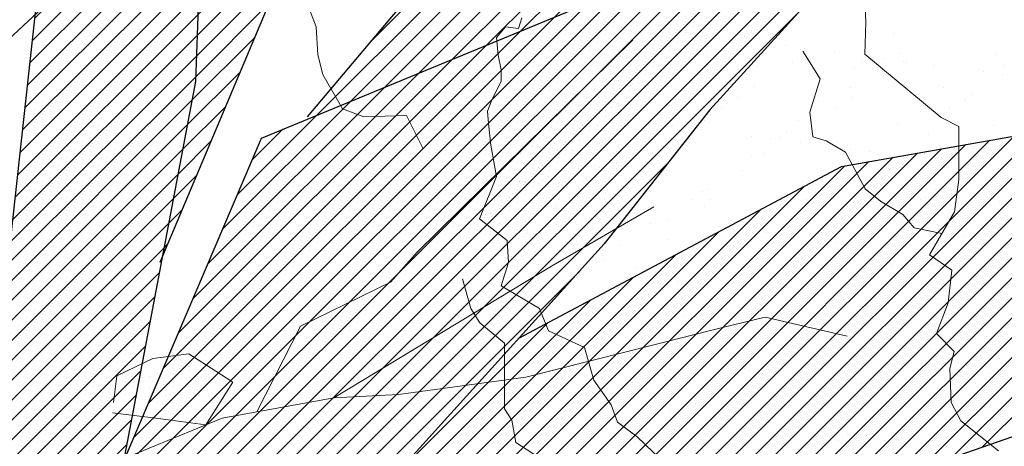
# Model space of a CAD drawing. Units: inches. Extents: x 1986 to 21484, y -1816 to 2016.
# Tile 32 of 85: x 2172.01 to 2182.74, y 1887.36 to 1892.02. Entities that reach past the tile are written whole.
import ezdxf

# ---------------------------------------------------------------- set-up
doc = ezdxf.new("R2010")
doc.units = ezdxf.units.IN
doc.layers.add('L-PLNT', color=84, linetype='Continuous', lineweight=13)
doc.layers.add('vfolhas', color=114, linetype='Continuous', lineweight=5)
doc.layers.add('vfolha2', color=110, linetype='Continuous')
doc.layers.add('vfolhas2', color=102, linetype='Continuous')
pattern_1 = [(45, (-2446.5133113, 50.986076), (-0.004419417382, 0.004419417382), [])]

# ---------------------------------------------------------------- blocks, each defined once
blk = doc.blocks.new('arbusto_PB_verde_grande')
at = {"layer": 'vfolha2'}
h = blk.add_hatch(dxfattribs=at)
h.set_pattern_fill('ANSI31', color=256, scale=0.05, style=0)
h.set_pattern_definition(pattern_1)
h.paths.add_polyline_path([(0.02944, 0.35651), (0.00028, 0.09048), (0.02625, -0.03934), (0.047, 0.06233), (0.06189, 0.09731), (0.09372, 0.26573), (0.09955, 0.43473), (0.08789, 0.61313), (0.0645, 0.72266), (0.04988, 0.6851), (0.0236, 0.51294)])
h.paths.add_polyline_path([(0.30106, 0.43789), (0.14225, 0.24871), (0.26685, 0.30022)])
h.paths.add_polyline_path([(0.37995, 0.22817), (0.23697, 0.15193), (0.18428, 0.09364), (0.11122, 0.04358), (0.02625, -0.03934), (0.28061, 0.04667), (0.36829, 0.07798), (0.46756, 0.11239), (0.61068, 0.19376), (0.71585, 0.27823), (0.55813, 0.25948)])
h.paths.add_polyline_path([(0.56101, -0.29441), (0.72752, -0.32573), (0.59024, -0.2412), (0.42962, -0.15982), (0.02625, -0.03934), (0.14922, -0.14107), (0.18838, -0.16604), (0.41501, -0.24435)])
h.paths.add_polyline_path([(-0.27429, -0.44776), (-0.30352, -0.72628), (-0.23923, -0.64175), (-0.15457, -0.45716), (0.02625, -0.03934), (-0.16328, -0.25376)])
h.paths.add_polyline_path([(-0.51963, -0.24744), (-0.67736, -0.32573), (-0.59558, -0.35072), (-0.40574, -0.32882), (-0.21007, -0.20995), (0.02625, -0.03934), (-0.14874, -0.06595), (-0.31518, -0.09101), (-0.41452, -0.15048)])
h.paths.add_polyline_path([(-0.52546, 0.25007), (-0.70947, 0.24698), (-0.51963, 0.1093), (-0.32979, 0.02167), (-0.07567, -0.0128), (-0.04234, -0.02148), (-0.35024, 0.1312)])
at = {"layer": 'vfolhas'}
h = blk.add_hatch(dxfattribs=at)
h.set_pattern_fill('ANSI31', color=256, scale=0.05, style=0)
h.set_pattern_definition(pattern_1)
h.paths.add_polyline_path([(-0.07279, 0.50669), (-0.18085, 0.65063), (-0.2334, 0.67253), (-0.20712, 0.53176), (-0.10785, 0.25007), (0.02625, -0.03934), (0.00028, 0.09048), (0.00816, 0.16241), (-0.04939, 0.29079)])
h.paths.add_polyline_path([(0.09902, 0.41929), (0.09372, 0.26573), (0.07906, 0.18814), (0.15506, 0.36901), (0.26606, 0.5505), (0.28356, 0.63504), (0.2485, 0.68819), (0.25145, 0.63504), (0.20178, 0.54426)])
h.paths.add_polyline_path([(0.12295, 0.24073), (0.047, 0.06233), (0.02625, -0.03934), (0.11122, 0.04358), (0.18428, 0.09364), (0.27478, 0.19376), (0.3215, 0.25323), (0.44129, 0.38467), (0.47634, 0.57866), (0.41789, 0.45347), (0.28939, 0.30954)])
h.paths.add_polyline_path([(0.58145, -0.03779), (0.70707, 0.01536), (0.78591, 0.04667), (0.74796, 0.06549), (0.62818, 0.08423), (0.52595, 0.09048), (0.39745, 0.04358), (0.02625, -0.03934), (0.25728, -0.03154), (0.43834, -0.0347)])
h.paths.add_polyline_path([(0.52022, -0.03647), (0.43834, -0.0347), (0.25728, -0.03154), (0.02625, -0.03934), (0.17964, -0.08515), (0.53768, -0.13167), (0.69541, -0.15357), (0.78591, -0.07852), (0.70413, -0.10042)])
h.paths.add_polyline_path([(0.27189, -0.21929), (0.14922, -0.14107), (0.02625, -0.03934), (0.15794, -0.31007), (0.29522, -0.42585), (0.41789, -0.49157), (0.56396, -0.56669), (0.5114, -0.48532), (0.39456, -0.34139)])
h.paths.add_polyline_path([(-0.05818, -0.47591), (-0.02312, -0.61984), (0.047, -0.80134), (0.08494, -0.59794), (0.07911, -0.4071), (0.03527, -0.25376), (0.02625, -0.03934), (-0.03773, -0.26001)])
h.paths.add_polyline_path([(-0.24218, 0.14054), (-0.11073, 0.06858), (0.02625, -0.03934), (-0.04235, 0.10871), (-0.21007, 0.23757), (-0.36485, 0.33145), (-0.47874, 0.40341), (-0.54303, 0.46288), (-0.49041, 0.33145), (-0.39408, 0.22192)])
at = {"layer": 'vfolha2'}
for p, q in [((0.14339, 0.25007), (0.30106, 0.43789)), ((0.09955, 0.43473), (0.09372, 0.26573)), ((0.00028, 0.09048), (0.02944, 0.35651)), ((0.37995, 0.22817), (0.55813, 0.25948)), ((0.23697, 0.15193), (0.37995, 0.22817))]:
    blk.add_line(p, q, dxfattribs=at)
at = {"layer": 'vfolhas2'}
for p, q in [((0.44129, 0.38467), (0.3215, 0.25323)), ((0.15506, 0.36901), (0.07795, 0.18551)), ((0.12295, 0.24073), (0.28939, 0.30954)), ((0.09372, 0.26573), (0.06189, 0.09731)), ((0.3215, 0.25323), (0.27478, 0.19376)), ((0.047, 0.06233), (0.12295, 0.24073)), ((0.27478, 0.19376), (0.18428, 0.09364)), ((0.46756, 0.11239), (0.36829, 0.07798))]:
    blk.add_line(p, q, dxfattribs=at)
blk = doc.blocks.new('PLANT-SHRUB')
for p, q in [((2171.837, 1891.752), (2172.54, 1892.411)), ((2175.047, 1892.46), (2175.244, 1891.941)), ((2181.225, 1892.278), (2181.234, 1891.991)), ((2177.484, 1892.037), (2177.448, 1891.922)), ((2178.209, 1892.018), (2178.209, 1892.018)), ((2178.417, 1891.991), (2178.417, 1891.991)), ((2178.742, 1891.948), (2178.742, 1891.948)), ((2181.234, 1891.991), (2181.225, 1891.643)), ((2175.244, 1891.941), (2175.262, 1891.636)), ((2177.307, 1891.939), (2177.209, 1891.824)), ((2177.448, 1891.922), (2177.307, 1891.939)), ((2178.292, 1891.909), (2178.292, 1891.909)), ((2178.568, 1891.93), (2178.568, 1891.93)), ((2178.681, 1891.891), (2178.681, 1891.891)), ((2178.722, 1891.865), (2178.722, 1891.865)), ((2178.789, 1891.908), (2178.789, 1891.908)), ((2179.285, 1891.877), (2179.285, 1891.877)), ((2179.493, 1891.849), (2179.493, 1891.849)), ((2179.91, 1891.837), (2179.91, 1891.837)), ((2179.984, 1891.904), (2179.984, 1891.904)), ((2181.533, 1891.872), (2181.533, 1891.872)), ((2176.344, 1889.483), (2178.697, 1891.799)), ((2177.209, 1891.824), (2177.227, 1891.63)), ((2178.689, 1891.748), (2178.689, 1891.748)), ((2179.818, 1891.807), (2179.818, 1891.807)), ((2180.361, 1891.735), (2180.361, 1891.735)), ((2175.262, 1891.636), (2175.316, 1891.422)), ((2177.227, 1891.63), (2177.262, 1891.471)), ((2178.558, 1891.622), (2178.558, 1891.622)), ((2179.503, 1891.686), (2179.503, 1891.686)), ((2180.525, 1891.691), (2180.525, 1891.691)), ((2180.736, 1891.375), (2180.547, 1891.676)), ((2180.569, 1891.708), (2180.569, 1891.708)), ((2180.894, 1891.665), (2180.894, 1891.665)), ((2181.225, 1891.643), (2182.057, 1890.952)), ((2181.604, 1891.652), (2181.604, 1891.652)), ((2182.651, 1891.639), (2182.651, 1891.639)), ((2179.193, 1891.557), (2179.193, 1891.557)), ((2180.438, 1891.555), (2180.438, 1891.555)), ((2181.185, 1891.553), (2181.185, 1891.553)), ((2181.437, 1891.593), (2181.437, 1891.593)), ((2181.645, 1891.566), (2181.645, 1891.566)), ((2181.682, 1891.553), (2181.682, 1891.553)), ((2181.97, 1891.523), (2181.97, 1891.523)), ((2182.734, 1891.521), (2182.734, 1891.521)), ((2175.316, 1891.422), (2175.531, 1891.046)), ((2177.262, 1891.471), (2177.262, 1891.347)), ((2178.593, 1891.464), (2178.593, 1891.464)), ((2178.66, 1891.507), (2178.66, 1891.507)), ((2178.764, 1891.464), (2178.764, 1891.464)), ((2179.512, 1891.472), (2179.512, 1891.472)), ((2181.112, 1891.486), (2181.112, 1891.486)), ((2182.512, 1891.452), (2182.512, 1891.452)), ((2182.72, 1891.424), (2182.72, 1891.424)), ((2177.262, 1891.347), (2177.156, 1891.135)), ((2178.328, 1891.382), (2178.328, 1891.382)), ((2178.411, 1891.371), (2178.411, 1891.371)), ((2178.541, 1891.354), (2178.541, 1891.354)), ((2178.548, 1891.314), (2178.548, 1891.314)), ((2178.694, 1891.323), (2178.694, 1891.323)), ((2178.758, 1891.325), (2178.758, 1891.325)), ((2178.938, 1891.33), (2178.938, 1891.33)), ((2180.625, 1891.008), (2180.736, 1891.375)), ((2178.276, 1891.262), (2178.276, 1891.262)), ((2178.665, 1891.296), (2178.665, 1891.296)), ((2180.018, 1891.291), (2180.018, 1891.291)), ((2181.064, 1891.278), (2181.064, 1891.278)), ((2182.086, 1891.282), (2182.086, 1891.282)), ((2182.387, 1891.202), (2182.387, 1891.202)), ((2177.156, 1891.135), (2177.112, 1891.02)), ((2178.033, 1891.108), (2178.033, 1891.108)), ((2178.322, 1891.171), (2178.322, 1891.171)), ((2178.506, 1891.151), (2178.506, 1891.151)), ((2178.531, 1891.107), (2178.531, 1891.107)), ((2179.091, 1891.086), (2179.091, 1891.086)), ((2179.165, 1891.153), (2179.165, 1891.153)), ((2179.831, 1891.169), (2179.831, 1891.169)), ((2180.714, 1891.121), (2180.714, 1891.121)), ((2181.076, 1891.166), (2181.076, 1891.166)), ((2182.313, 1891.135), (2182.313, 1891.135)), ((2182.32, 1891.164), (2182.32, 1891.164)), ((2175.531, 1891.046), (2175.764, 1890.957)), ((2177.112, 1891.02), (2177.121, 1890.887)), ((2177.963, 1891.016), (2177.963, 1891.016)), ((2177.966, 1891.065), (2177.966, 1891.065)), ((2178.119, 1891.011), (2178.119, 1891.011)), ((2178.181, 1890.987), (2178.181, 1890.987)), ((2178.264, 1890.976), (2178.264, 1890.976)), ((2178.337, 1890.996), (2178.337, 1890.996)), ((2178.367, 1891.023), (2178.367, 1891.023)), ((2178.464, 1891.064), (2178.464, 1891.064)), ((2178.537, 1891.006), (2178.537, 1891.006)), ((2179.662, 1891.061), (2179.662, 1891.061)), ((2180.658, 1890.74), (2180.625, 1891.008)), ((2180.907, 1891.059), (2180.907, 1891.059)), ((2182.152, 1891.057), (2182.152, 1891.057)), ((2175.764, 1890.957), (2176.229, 1890.974)), ((2176.229, 1890.974), (2176.408, 1890.617)), ((2176.229, 1890.974), (2176.229, 1890.974)), ((2177.121, 1890.887), (2177.147, 1890.649)), ((2178.394, 1890.959), (2178.394, 1890.959)), ((2178.611, 1890.931), (2178.611, 1890.931)), ((2178.916, 1890.89), (2178.916, 1890.89)), ((2179.477, 1890.916), (2179.477, 1890.916)), ((2180.5, 1890.921), (2180.5, 1890.921)), ((2181.579, 1890.882), (2181.579, 1890.882)), ((2182.057, 1890.952), (2182.25, 1890.855)), ((2182.625, 1890.869), (2182.625, 1890.869)), ((2177.903, 1890.861), (2177.903, 1890.861)), ((2178.147, 1890.862), (2178.147, 1890.862)), ((2178.178, 1890.85), (2178.178, 1890.85)), ((2178.312, 1890.863), (2178.312, 1890.863)), ((2178.645, 1890.861), (2178.645, 1890.861)), ((2179.125, 1890.863), (2179.125, 1890.863)), ((2179.449, 1890.82), (2179.449, 1890.82)), ((2180.366, 1890.803), (2180.366, 1890.803)), ((2181.915, 1890.77), (2181.915, 1890.77)), ((2182.25, 1890.855), (2182.25, 1890.276)), ((2177.677, 1890.719), (2177.677, 1890.719)), ((2177.837, 1890.665), (2177.837, 1890.665)), ((2177.904, 1890.708), (2177.904, 1890.708)), ((2178.01, 1890.696), (2178.01, 1890.696)), ((2178.039, 1890.723), (2178.039, 1890.723)), ((2178.109, 1890.703), (2178.109, 1890.703)), ((2178.335, 1890.664), (2178.335, 1890.664)), ((2178.402, 1890.707), (2178.402, 1890.707)), ((2178.527, 1890.698), (2178.527, 1890.698)), ((2178.693, 1890.721), (2178.693, 1890.721)), ((2179.992, 1890.749), (2179.992, 1890.749)), ((2180.2, 1890.721), (2180.2, 1890.721)), ((2180.292, 1890.735), (2180.292, 1890.735)), ((2180.525, 1890.679), (2180.525, 1890.679)), ((2180.803, 1890.696), (2180.658, 1890.74)), ((2181.015, 1890.573), (2180.803, 1890.696)), ((2177.147, 1890.649), (2177.209, 1890.308)), ((2177.474, 1890.559), (2177.474, 1890.559)), ((2177.603, 1890.649), (2177.603, 1890.649)), ((2177.686, 1890.639), (2177.686, 1890.639)), ((2177.816, 1890.621), (2177.816, 1890.621)), ((2177.851, 1890.55), (2177.851, 1890.55)), ((2177.893, 1890.553), (2177.893, 1890.553)), ((2178.033, 1890.593), (2178.033, 1890.593)), ((2178.116, 1890.582), (2178.116, 1890.582)), ((2178.246, 1890.565), (2178.246, 1890.565)), ((2178.302, 1890.555), (2178.302, 1890.555)), ((2178.49, 1890.556), (2178.49, 1890.556)), ((2178.52, 1890.583), (2178.52, 1890.583)), ((2178.87, 1890.557), (2178.87, 1890.557)), ((2178.913, 1890.56), (2178.913, 1890.56)), ((2180.115, 1890.554), (2180.115, 1890.554)), ((2181.115, 1890.384), (2181.015, 1890.573)), ((2181.068, 1890.607), (2181.068, 1890.607)), ((2181.276, 1890.58), (2181.276, 1890.58)), ((2181.36, 1890.552), (2181.36, 1890.552)), ((2182.604, 1890.55), (2182.604, 1890.55)), ((2177.52, 1890.463), (2177.52, 1890.463)), ((2178.018, 1890.462), (2178.018, 1890.462)), ((2178.464, 1890.536), (2178.464, 1890.536)), ((2178.516, 1890.461), (2178.516, 1890.461)), ((2178.547, 1890.525), (2178.547, 1890.525)), ((2179.993, 1890.521), (2179.993, 1890.521)), ((2181.039, 1890.507), (2181.039, 1890.507)), ((2181.568, 1890.452), (2181.568, 1890.452)), ((2181.601, 1890.537), (2181.601, 1890.537)), ((2182.061, 1890.512), (2182.061, 1890.512)), ((2182.144, 1890.466), (2182.144, 1890.466)), ((2177.667, 1890.411), (2177.667, 1890.411)), ((2177.682, 1890.396), (2177.682, 1890.396)), ((2177.711, 1890.423), (2177.711, 1890.423)), ((2178.099, 1890.395), (2178.099, 1890.395)), ((2178.331, 1890.41), (2178.331, 1890.41)), ((2178.517, 1890.39), (2178.517, 1890.39)), ((2179.895, 1890.371), (2179.895, 1890.371)), ((2181.226, 1890.172), (2181.115, 1890.384)), ((2181.494, 1890.384), (2181.494, 1890.384)), ((2182.352, 1890.438), (2182.352, 1890.438)), ((2182.677, 1890.395), (2182.677, 1890.395)), ((2177.209, 1890.308), (2177.023, 1889.848)), ((2177.21, 1890.265), (2177.21, 1890.265)), ((2177.238, 1890.284), (2177.238, 1890.284)), ((2177.277, 1890.308), (2177.277, 1890.308)), ((2177.456, 1890.255), (2177.456, 1890.255)), ((2177.464, 1890.251), (2177.464, 1890.251)), ((2177.523, 1890.25), (2177.523, 1890.25)), ((2177.539, 1890.244), (2177.539, 1890.244)), ((2177.669, 1890.227), (2177.669, 1890.227)), ((2177.708, 1890.264), (2177.708, 1890.264)), ((2177.775, 1890.307), (2177.775, 1890.307)), ((2177.883, 1890.245), (2177.883, 1890.245)), ((2178.163, 1890.255), (2178.163, 1890.255)), ((2178.192, 1890.282), (2178.192, 1890.282)), ((2178.206, 1890.263), (2178.206, 1890.263)), ((2178.273, 1890.306), (2178.273, 1890.306)), ((2178.292, 1890.247), (2178.292, 1890.247)), ((2182.25, 1890.276), (2182.202, 1889.922)), ((2182.25, 1890.276), (2182.25, 1890.276)), ((2177.384, 1890.122), (2177.384, 1890.122)), ((2177.886, 1890.198), (2177.886, 1890.198)), ((2177.969, 1890.187), (2177.969, 1890.187)), ((2178.099, 1890.17), (2178.099, 1890.17)), ((2178.316, 1890.142), (2178.316, 1890.142)), ((2178.399, 1890.131), (2178.399, 1890.131)), ((2179.452, 1890.146), (2179.452, 1890.146)), ((2179.508, 1890.168), (2179.508, 1890.168)), ((2180.475, 1890.151), (2180.475, 1890.151)), ((2180.753, 1890.166), (2180.753, 1890.166)), ((2181.394, 1890.039), (2181.226, 1890.172)), ((2181.997, 1890.163), (2181.997, 1890.163)), ((2177.248, 1890.101), (2177.248, 1890.101)), ((2177.354, 1890.095), (2177.354, 1890.095)), ((2177.391, 1890.062), (2177.391, 1890.062)), ((2177.657, 1890.103), (2177.657, 1890.103)), ((2177.889, 1890.061), (2177.889, 1890.061)), ((2178.003, 1890.109), (2178.003, 1890.109)), ((2178.089, 1890.087), (2178.089, 1890.087)), ((2178.387, 1890.061), (2178.387, 1890.061)), ((2179.34, 1890.06), (2179.34, 1890.06)), ((2179.547, 1890.052), (2179.547, 1890.052)), ((2180.584, 1890.058), (2180.584, 1890.058)), ((2181.096, 1890.02), (2181.096, 1890.02)), ((2181.639, 1889.894), (2181.394, 1890.039)), ((2181.554, 1890.112), (2181.554, 1890.112)), ((2181.829, 1890.056), (2181.829, 1890.056)), ((2182.6, 1890.099), (2182.6, 1890.099)), ((2182.695, 1890.034), (2182.695, 1890.034)), ((2177.148, 1889.908), (2177.148, 1889.908)), ((2177.195, 1889.95), (2177.195, 1889.95)), ((2177.454, 1889.943), (2177.454, 1889.943)), ((2177.646, 1889.907), (2177.646, 1889.907)), ((2177.827, 1889.339), (2178.923, 1889.978)), ((2177.835, 1889.955), (2177.835, 1889.955)), ((2177.864, 1889.982), (2177.864, 1889.982)), ((2177.873, 1889.937), (2177.873, 1889.937)), ((2178.144, 1889.906), (2178.144, 1889.906)), ((2178.282, 1889.939), (2178.282, 1889.939)), ((2178.548, 1889.904), (2178.548, 1889.904)), ((2179.473, 1889.984), (2179.473, 1889.984)), ((2182.202, 1889.922), (2181.928, 1889.454)), ((2177.023, 1889.848), (2177.324, 1889.61)), ((2177.056, 1889.822), (2177.056, 1889.822)), ((2177.081, 1889.865), (2177.081, 1889.865)), ((2177.091, 1889.889), (2177.091, 1889.889)), ((2177.308, 1889.86), (2177.308, 1889.86)), ((2177.391, 1889.849), (2177.391, 1889.849)), ((2177.521, 1889.832), (2177.521, 1889.832)), ((2178.077, 1889.863), (2178.077, 1889.863)), ((2178.316, 1889.815), (2178.316, 1889.815)), ((2178.345, 1889.842), (2178.345, 1889.842)), ((2178.756, 1889.877), (2178.756, 1889.877)), ((2179.081, 1889.834), (2179.081, 1889.834)), ((2181.761, 1889.749), (2181.639, 1889.894)), ((2177.238, 1889.793), (2177.238, 1889.793)), ((2177.866, 1889.785), (2177.866, 1889.785)), ((2178.079, 1889.779), (2178.079, 1889.779)), ((2178.169, 1889.747), (2178.169, 1889.747)), ((2178.252, 1889.736), (2178.252, 1889.736)), ((2178.382, 1889.719), (2178.382, 1889.719)), ((2178.888, 1889.79), (2178.888, 1889.79)), ((2179.624, 1889.763), (2179.624, 1889.763)), ((2179.832, 1889.735), (2179.832, 1889.735)), ((2179.968, 1889.751), (2179.968, 1889.751)), ((2180.157, 1889.692), (2180.157, 1889.692)), ((2180.748, 1889.701), (2180.748, 1889.701)), ((2181.014, 1889.737), (2181.014, 1889.737)), ((2182.065, 1889.688), (2181.761, 1889.749)), ((2182.036, 1889.742), (2182.036, 1889.742)), ((2177.262, 1889.662), (2177.262, 1889.662)), ((2177.324, 1889.61), (2177.341, 1889.371)), ((2177.444, 1889.635), (2177.444, 1889.635)), ((2177.507, 1889.655), (2177.507, 1889.655)), ((2177.537, 1889.682), (2177.537, 1889.682)), ((2179.075, 1889.62), (2179.075, 1889.62)), ((2180.675, 1889.634), (2180.675, 1889.634)), ((2180.7, 1889.621), (2180.7, 1889.621)), ((2180.908, 1889.593), (2180.908, 1889.593)), ((2182.298, 1889.669), (2182.298, 1889.669)), ((2176.055, 1889.155), (2176.344, 1889.483)), ((2177.348, 1889.509), (2177.348, 1889.509)), ((2177.517, 1889.507), (2177.517, 1889.507)), ((2177.637, 1889.487), (2177.637, 1889.487)), ((2178.548, 1889.556), (2178.548, 1889.556)), ((2179.792, 1889.554), (2179.792, 1889.554)), ((2181.037, 1889.551), (2181.037, 1889.551)), ((2181.233, 1889.551), (2181.233, 1889.551)), ((2181.775, 1889.479), (2181.775, 1889.479)), ((2182.281, 1889.549), (2182.281, 1889.549)), ((2177.341, 1889.371), (2177.262, 1889.115)), ((2177.374, 1889.438), (2177.374, 1889.438)), ((2177.45, 1889.464), (2177.45, 1889.464)), ((2177.591, 1889.409), (2177.591, 1889.409)), ((2177.674, 1889.398), (2177.674, 1889.398)), ((2178.381, 1889.389), (2178.381, 1889.389)), ((2179.427, 1889.376), (2179.427, 1889.376)), ((2180.449, 1889.381), (2180.449, 1889.381)), ((2181.928, 1889.454), (2182.173, 1889.288)), ((2181.983, 1889.452), (2181.983, 1889.452)), ((2182.308, 1889.409), (2182.308, 1889.409)), ((2175.438, 1887.895), (2177.827, 1889.339)), ((2177.434, 1889.327), (2177.434, 1889.327)), ((2177.631, 1889.261), (2177.631, 1889.261)), ((2178.728, 1889.301), (2178.728, 1889.301)), ((2180.277, 1889.269), (2180.277, 1889.269)), ((2181.529, 1889.342), (2181.529, 1889.342)), ((2181.876, 1889.283), (2181.876, 1889.283)), ((2181.95, 1889.35), (2181.95, 1889.35)), ((2182.173, 1889.288), (2182.133, 1888.93)), ((2182.575, 1889.329), (2182.575, 1889.329)), ((2175.073, 1888.674), (2176.055, 1889.155)), ((2176.839, 1889.192), (2176.839, 1889.192)), ((2176.928, 1888.868), (2176.839, 1889.192)), ((2177.941, 1889.169), (2177.941, 1889.169)), ((2178.654, 1889.234), (2178.654, 1889.234)), ((2179.185, 1889.167), (2179.185, 1889.167)), ((2180.43, 1889.165), (2180.43, 1889.165)), ((2181.675, 1889.163), (2181.675, 1889.163)), ((2177.262, 1889.115), (2177.677, 1888.868)), ((2177.262, 1889.115), (2177.262, 1889.115)), ((2177.388, 1889.106), (2177.388, 1889.106)), ((2179.017, 1889.06), (2179.017, 1889.06)), ((2180.262, 1889.057), (2180.262, 1889.057)), ((2181.506, 1889.055), (2181.506, 1889.055)), ((2177.84, 1889.015), (2177.84, 1889.015)), ((2178.863, 1889.02), (2178.863, 1889.02)), ((2179.929, 1888.951), (2179.929, 1888.951)), ((2179.942, 1888.981), (2179.942, 1888.981)), ((2180.989, 1888.967), (2180.989, 1888.967)), ((2182.011, 1888.972), (2182.011, 1888.972)), ((2177.029, 1888.712), (2176.928, 1888.868)), ((2177.677, 1888.868), (2177.778, 1888.623)), ((2178.179, 1888.918), (2178.179, 1888.918)), ((2178.256, 1888.869), (2178.256, 1888.869)), ((2178.388, 1888.89), (2178.388, 1888.89)), ((2178.712, 1888.848), (2178.712, 1888.848)), ((2179.856, 1888.883), (2179.856, 1888.883)), ((2181.478, 1888.918), (2181.478, 1888.918)), ((2182.133, 1888.93), (2182.006, 1888.597)), ((2179.255, 1888.776), (2179.255, 1888.776)), ((2179.463, 1888.749), (2179.463, 1888.749)), ((2179.642, 1888.652), (2180.139, 1888.772)), ((2180.139, 1888.772), (2181.03, 1888.566)), ((2174.599, 1887.742), (2175.073, 1888.674)), ((2177.297, 1888.489), (2177.029, 1888.712)), ((2177.529, 1888.118), (2179.642, 1888.652)), ((2177.778, 1888.623), (2178.169, 1888.444)), ((2178.356, 1888.619), (2178.356, 1888.619)), ((2179.788, 1888.706), (2179.788, 1888.706)), ((2180.331, 1888.635), (2180.331, 1888.635)), ((2178.225, 1888.555), (2178.225, 1888.555)), ((2179.402, 1888.606), (2179.402, 1888.606)), ((2179.458, 1888.519), (2179.458, 1888.519)), ((2179.469, 1888.553), (2179.469, 1888.553)), ((2180.424, 1888.611), (2180.424, 1888.611)), ((2180.539, 1888.607), (2180.539, 1888.607)), ((2180.714, 1888.55), (2180.714, 1888.55)), ((2180.864, 1888.564), (2180.864, 1888.564)), ((2181.057, 1888.532), (2181.057, 1888.532)), ((2181.131, 1888.6), (2181.131, 1888.6)), ((2181.504, 1888.572), (2181.504, 1888.572)), ((2181.959, 1888.548), (2181.959, 1888.548)), ((2182.006, 1888.597), (2182.197, 1888.398)), ((2182.55, 1888.559), (2182.55, 1888.559)), ((2182.68, 1888.568), (2182.68, 1888.568)), ((2177.297, 1888.198), (2177.297, 1888.489)), ((2178.169, 1888.444), (2178.27, 1888.086)), ((2178.169, 1888.444), (2178.169, 1888.444)), ((2181.407, 1888.493), (2181.407, 1888.493)), ((2181.615, 1888.466), (2181.615, 1888.466)), ((2181.94, 1888.423), (2181.94, 1888.423)), ((2173.071, 1888.134), (2173.464, 1888.322)), ((2173.464, 1888.322), (2173.858, 1888.374)), ((2173.621, 1888.305), (2173.621, 1888.305)), ((2173.727, 1888.316), (2173.727, 1888.316)), ((2173.858, 1888.374), (2174.149, 1888.186)), ((2173.858, 1888.374), (2173.858, 1888.374)), ((2173.858, 1888.374), (2173.858, 1888.374)), ((2182.197, 1888.398), (2182.149, 1888.215)), ((2182.483, 1888.351), (2182.483, 1888.351)), ((2182.691, 1888.324), (2182.691, 1888.324)), ((2173.848, 1888.234), (2173.848, 1888.234)), ((2173.885, 1888.268), (2173.885, 1888.268)), ((2174.149, 1888.186), (2174.337, 1888.066)), ((2177.297, 1887.774), (2177.297, 1888.198)), ((2178.838, 1888.249), (2178.838, 1888.249)), ((2179.11, 1888.2), (2179.11, 1888.2)), ((2179.917, 1888.211), (2179.917, 1888.211)), ((2180.963, 1888.197), (2180.963, 1888.197)), ((2181.986, 1888.202), (2181.986, 1888.202)), ((2182.149, 1888.215), (2182.165, 1887.842)), ((2182.332, 1888.249), (2182.332, 1888.249)), ((2173.036, 1887.844), (2173.071, 1888.134)), ((2173.071, 1888.134), (2173.071, 1888.134)), ((2173.351, 1888.118), (2173.351, 1888.118)), ((2173.423, 1888.123), (2173.423, 1888.123)), ((2173.862, 1888.12), (2173.862, 1888.12)), ((2174.046, 1888.122), (2174.046, 1888.122)), ((2176.141, 1887.929), (2177.529, 1888.118)), ((2178.27, 1888.086), (2178.46, 1887.818)), ((2178.863, 1888.166), (2178.863, 1888.166)), ((2179.036, 1888.132), (2179.036, 1888.132)), ((2180.107, 1888.164), (2180.107, 1888.164)), ((2180.659, 1888.168), (2180.659, 1888.168)), ((2181.352, 1888.162), (2181.352, 1888.162)), ((2182.258, 1888.182), (2182.258, 1888.182)), ((2182.597, 1888.159), (2182.597, 1888.159)), ((2173.156, 1888.027), (2173.156, 1888.027)), ((2173.339, 1888.069), (2173.339, 1888.069)), ((2173.427, 1887.991), (2173.427, 1887.991)), ((2173.531, 1887.978), (2173.531, 1887.978)), ((2173.649, 1888.052), (2173.649, 1888.052)), ((2173.961, 1888.068), (2173.961, 1888.068)), ((2174.337, 1888.066), (2174.043, 1887.599)), ((2174.337, 1888.066), (2174.337, 1888.066)), ((2178.694, 1888.059), (2178.694, 1888.059)), ((2179.939, 1888.057), (2179.939, 1888.057)), ((2181.183, 1888.054), (2181.183, 1888.054)), ((2182.428, 1888.052), (2182.428, 1888.052)), ((2173.069, 1887.94), (2173.069, 1887.94)), ((2173.475, 1887.893), (2173.475, 1887.893)), ((2173.609, 1887.92), (2173.609, 1887.92)), ((2173.694, 1887.956), (2173.694, 1887.956)), ((2173.965, 1887.92), (2173.965, 1887.92)), ((2174.069, 1887.907), (2174.069, 1887.907)), ((2174.132, 1887.913), (2174.132, 1887.913)), ((2174.221, 1887.672), (2175.438, 1887.895)), ((2175.438, 1887.895), (2176.141, 1887.929)), ((2173.439, 1887.859), (2173.439, 1887.859)), ((2173.565, 1887.816), (2173.565, 1887.816)), ((2177.375, 1887.651), (2177.297, 1887.774)), ((2178.46, 1887.818), (2178.527, 1887.628)), ((2178.887, 1887.79), (2178.887, 1887.79)), ((2179.095, 1887.763), (2179.095, 1887.763)), ((2179.377, 1887.836), (2179.377, 1887.836)), ((2180.238, 1887.782), (2180.238, 1887.782)), ((2180.311, 1887.849), (2180.311, 1887.849)), ((2180.399, 1887.841), (2180.399, 1887.841)), ((2181.479, 1887.802), (2181.479, 1887.802)), ((2181.861, 1887.817), (2181.861, 1887.817)), ((2182.165, 1887.842), (2182.269, 1887.643)), ((2182.525, 1887.788), (2182.525, 1887.788)), ((2172.884, 1887.124), (2174.221, 1887.672)), ((2173.498, 1887.673), (2173.023, 1887.729)), ((2173.338, 1887.733), (2173.338, 1887.733)), ((2174.043, 1887.599), (2173.498, 1887.673)), ((2173.849, 1887.735), (2173.849, 1887.735)), ((2174.039, 1887.684), (2174.039, 1887.684)), ((2174.076, 1887.717), (2174.076, 1887.717)), ((2177.42, 1887.405), (2177.375, 1887.651)), ((2179.42, 1887.72), (2179.42, 1887.72)), ((2173.884, 1887.621), (2173.884, 1887.621)), ((2178.527, 1887.628), (2178.739, 1887.472)), ((2179.147, 1887.552), (2179.147, 1887.552)), ((2179.963, 1887.648), (2179.963, 1887.648)), ((2180.171, 1887.621), (2180.171, 1887.621)), ((2180.391, 1887.55), (2180.391, 1887.55)), ((2180.496, 1887.578), (2180.496, 1887.578)), ((2181.636, 1887.547), (2181.636, 1887.547)), ((2182.269, 1887.643), (2182.682, 1887.317)), ((2178.739, 1887.472), (2179.007, 1887.215)), ((2179.892, 1887.44), (2179.892, 1887.44)), ((2181.038, 1887.507), (2181.038, 1887.507)), ((2181.247, 1887.479), (2181.247, 1887.479)), ((2181.513, 1887.498), (2181.513, 1887.498)), ((2181.571, 1887.436), (2181.571, 1887.436)), ((2177.667, 1887.245), (2177.42, 1887.405)), ((2179.84, 1887.417), (2179.84, 1887.417)), ((2180.938, 1887.427), (2180.938, 1887.427)), ((2181.439, 1887.431), (2181.439, 1887.431)), ((2181.961, 1887.432), (2181.961, 1887.432)), ((2182.114, 1887.365), (2182.114, 1887.365))]:
    blk.add_line(p, q)

msp = doc.modelspace()

# ---------------------------------------------------------------- block references
at = {"layer": 'L-PLNT'}
msp.add_blockref('PLANT-SHRUB', (0, 0), dxfattribs=at)
at = {"layer": 'L-PLNT', "xscale": 24.60366729364114, "yscale": 24.60366729364114, "zscale": 24.60366729364114}
msp.add_blockref('arbusto_PB_verde_grande', (2171.623, 1884.805), dxfattribs=at)

doc.saveas('drawing.dxf')
